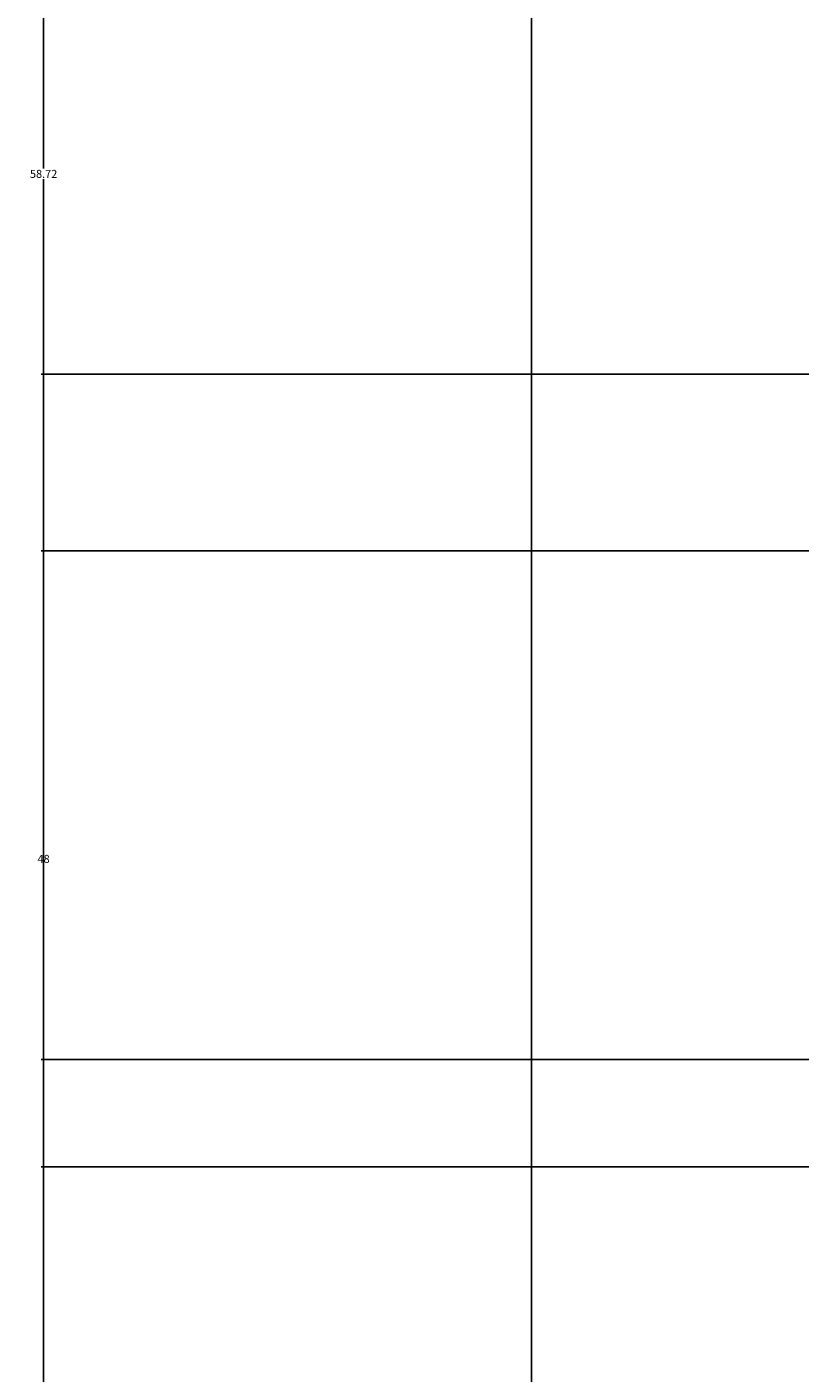
# Model space of a CAD drawing. Units: inches. Extents: x -13 to 809, y 112 to 656.
# Tile 26 of 55: x -13 to 47, y 446 to 551. Entities that reach past the tile are written whole.
import ezdxf

# ---------------------------------------------------------------- set-up
doc = ezdxf.new("R2010")
doc.units = ezdxf.units.IN
doc.header["$MEASUREMENT"] = 0
doc.layers.add('A-ANNO-DIMS', color=2, linetype='Continuous', lineweight=18)
doc.styles.get("Standard").update_dxf_attribs({"font": 'arial.ttf'})
doc.dimstyles.get("Standard").update_dxf_attribs({"dimtxt": 0.625, "dimasz": 0.18, "dimexe": 0.18, "dimexo": 0.0625, "dimgap": 0.09, "dimtad": 0, "dimtih": 1, "dimtoh": 1, "dimdec": 4, "dimzin": 0, "dimdsep": 46, "dimlunit": 4, "dimtxsty": 'Standard', "dimcen": 0.09, "dimadec": 0, "dimazin": 0, "dimtfac": 1, "dimtdec": 4, "dimtofl": 0, "dimtmove": 0, "dimatfit": 3, "dimfxl": 1, "dimtolj": 1, "dimtzin": 0, "dimarcsym": 0})

# ---------------------------------------------------------------- blocks, each defined once
blk = doc.blocks.new('*D22')
at = {"layer": 'A-ANNO-DIMS', "color": 0, "lineweight": -2, "transparency": 16777216}
for p, q in [((26.08, 210.58), (26.08, 655.96)), ((26.26, 655.78), (65.52, 655.78)), ((107.08, 655.78), (67.82, 655.78)), ((107.26, 510.58), (107.26, 655.96))]:
    blk.add_line(p, q, dxfattribs=at)
at = {"layer": 'A-ANNO-DIMS', "color": 0, "transparency": 16777216}
for points in [[(26.26, 655.81), (26.26, 655.75), (26.08, 655.78)], [(107.08, 655.81), (107.08, 655.75), (107.26, 655.78)]]:
    blk.add_solid(points, dxfattribs=at)
at = {"layer": 'Defpoints', "color": 0, "transparency": 16777216}
for p in [(107.26, 655.78), (107.26, 510.52), (26.08, 210.52)]:
    blk.add_point(p, dxfattribs=at)
at = {"layer": 'A-ANNO-DIMS', "color": 0, "transparency": 16777216, "insert": (66.67, 655.78), "char_height": 0.625, "attachment_point": 5}
blk.add_mtext('\\A1;81.18', dxfattribs=at)
blk = doc.blocks.new('*D34')
at = {"layer": 'A-ANNO-DIMS', "color": 0, "lineweight": -2, "transparency": 16777216}
for p, q in [((94.98, 462.52), (-12.1, 462.52)), ((-11.92, 462.34), (-11.92, 384.93)), ((-11.92, 306.7), (-11.92, 384.11)), ((94.98, 306.52), (-12.1, 306.52))]:
    blk.add_line(p, q, dxfattribs=at)
at = {"layer": 'A-ANNO-DIMS', "color": 0, "transparency": 16777216}
for points in [[(-11.95, 462.34), (-11.89, 462.34), (-11.92, 462.52)], [(-11.95, 306.7), (-11.89, 306.7), (-11.92, 306.52)]]:
    blk.add_solid(points, dxfattribs=at)
at = {"layer": 'Defpoints', "color": 0, "transparency": 16777216}
for p in [(-11.92, 462.52), (95.05, 462.52), (95.05, 306.52)]:
    blk.add_point(p, dxfattribs=at)
at = {"layer": 'A-ANNO-DIMS', "color": 0, "transparency": 16777216, "insert": (-11.92, 384.52), "char_height": 0.625, "attachment_point": 5}
blk.add_mtext('\\A1;156', dxfattribs=at)
blk = doc.blocks.new('*D35')
at = {"layer": 'A-ANNO-DIMS', "color": 0, "lineweight": -2, "transparency": 16777216}
for p, q in [((107.2, 510.52), (-12.1, 510.52)), ((-11.92, 510.34), (-11.92, 486.93)), ((-11.92, 462.7), (-11.92, 486.11)), ((107.2, 462.52), (-12.1, 462.52))]:
    blk.add_line(p, q, dxfattribs=at)
at = {"layer": 'A-ANNO-DIMS', "color": 0, "transparency": 16777216}
for points in [[(-11.95, 510.34), (-11.89, 510.34), (-11.92, 510.52)], [(-11.95, 462.7), (-11.89, 462.7), (-11.92, 462.52)]]:
    blk.add_solid(points, dxfattribs=at)
at = {"layer": 'Defpoints', "color": 0, "transparency": 16777216}
for p in [(-11.92, 510.52), (107.26, 510.52), (107.26, 462.52)]:
    blk.add_point(p, dxfattribs=at)
at = {"layer": 'A-ANNO-DIMS', "color": 0, "transparency": 16777216, "insert": (-11.92, 486.52), "char_height": 0.625, "attachment_point": 5}
blk.add_mtext('\\A1;48', dxfattribs=at)
blk = doc.blocks.new('*D36')
at = {"layer": 'A-ANNO-DIMS', "color": 0, "lineweight": -2, "transparency": 16777216}
for p, q in [((311.64, 569.24), (-12.1, 569.24)), ((-11.92, 569.06), (-11.92, 540.29)), ((-11.92, 510.7), (-11.92, 539.47)), ((107.2, 510.52), (-12.1, 510.52))]:
    blk.add_line(p, q, dxfattribs=at)
at = {"layer": 'A-ANNO-DIMS', "color": 0, "transparency": 16777216}
for points in [[(-11.95, 569.06), (-11.89, 569.06), (-11.92, 569.24)], [(-11.95, 510.7), (-11.89, 510.7), (-11.92, 510.52)]]:
    blk.add_solid(points, dxfattribs=at)
at = {"layer": 'Defpoints', "color": 0, "transparency": 16777216}
for p in [(-11.92, 569.24), (311.7, 569.24), (107.26, 510.52)]:
    blk.add_point(p, dxfattribs=at)
at = {"layer": 'A-ANNO-DIMS', "color": 0, "transparency": 16777216, "insert": (-11.92, 539.88), "char_height": 0.625, "attachment_point": 5}
blk.add_mtext('\\A1;58.72', dxfattribs=at)
blk = doc.blocks.new('*D39')
at = {"layer": 'A-ANNO-DIMS', "color": 0, "lineweight": -2, "transparency": 16777216}
for p, q in [((341.34, 524.28), (-12.1, 524.28)), ((-11.92, 524.1), (-11.92, 406.78)), ((-11.92, 288.63), (-11.92, 405.96)), ((341.34, 288.45), (-12.1, 288.45))]:
    blk.add_line(p, q, dxfattribs=at)
at = {"layer": 'A-ANNO-DIMS', "color": 0, "transparency": 16777216}
for points in [[(-11.95, 524.1), (-11.89, 524.1), (-11.92, 524.28)], [(-11.95, 288.63), (-11.89, 288.63), (-11.92, 288.45)]]:
    blk.add_solid(points, dxfattribs=at)
at = {"layer": 'Defpoints', "color": 0, "transparency": 16777216}
for p in [(-11.92, 524.28), (341.41, 524.28), (341.41, 288.45)]:
    blk.add_point(p, dxfattribs=at)
at = {"layer": 'A-ANNO-DIMS', "color": 0, "transparency": 16777216, "insert": (-11.92, 406.37), "char_height": 0.625, "attachment_point": 5}
blk.add_mtext('\\A1;235.83', dxfattribs=at)
blk = doc.blocks.new('*D43')
at = {"layer": 'A-ANNO-DIMS', "color": 0, "lineweight": -2, "transparency": 16777216}
for p, q in [((471.04, 470.88), (-12.1, 470.88)), ((-11.92, 470.7), (-11.92, 443.28)), ((-11.92, 415.04), (-11.92, 442.46)), ((471.04, 414.86), (-12.1, 414.86))]:
    blk.add_line(p, q, dxfattribs=at)
at = {"layer": 'A-ANNO-DIMS', "color": 0, "transparency": 16777216}
for points in [[(-11.95, 470.7), (-11.89, 470.7), (-11.92, 470.88)], [(-11.95, 415.04), (-11.89, 415.04), (-11.92, 414.86)]]:
    blk.add_solid(points, dxfattribs=at)
at = {"layer": 'Defpoints', "color": 0, "transparency": 16777216}
for p in [(-11.92, 470.88), (471.1, 470.88), (471.1, 414.86)]:
    blk.add_point(p, dxfattribs=at)
at = {"layer": 'A-ANNO-DIMS', "color": 0, "transparency": 16777216, "insert": (-11.92, 442.87), "char_height": 0.625, "attachment_point": 5}
blk.add_mtext('\\A1;56.02', dxfattribs=at)

msp = doc.modelspace()

# ---------------------------------------------------------------- dimensions: what is measured, and where the dimension line sits
at = {"layer": 'A-ANNO-DIMS'}
dim = msp.add_linear_dim(base=(107.2588, 655.7828), p1=(26.0809, 210.5199), p2=(107.2588, 510.5199), dimstyle='Standard', override={"dimdec": 2, "dimlfac": 1, "dimrnd": 0, "dimzin": 0, "dimdsep": 46, "dimlunit": 2}, dxfattribs=at)
dim.commit()
dim.dimension.update_dxf_attribs({"geometry": '*D22', "text_midpoint": (66.6698, 655.7828)})
for base, p1, p2, override, picture, middle in [((-11.9191, 569.2414), (107.2588, 510.5199), (311.6991, 569.2414), {"dimdec": 2, "dimlfac": 1, "dimrnd": 0, "dimzin": 0, "dimdsep": 46, "dimlunit": 2}, '*D36', (-11.9191, 539.8806)), ((-11.9191, 524.281), (341.4072, 288.4508), (341.4072, 524.281), {"dimdec": 2, "dimlfac": 1, "dimrnd": 0, "dimzin": 0, "dimdsep": 46, "dimlunit": 2}, '*D39', (-11.9191, 406.3659)), ((-11.9191, 510.5199), (107.2588, 462.5199), (107.2588, 510.5199), {"dimdec": 0, "dimlfac": 1, "dimrnd": 0, "dimzin": 0, "dimdsep": 46, "dimlunit": 2}, '*D35', (-11.9191, 486.5199)), ((-11.9191, 470.8765), (471.0998, 414.8594), (471.0998, 470.8765), {"dimdec": 2, "dimlfac": 1, "dimrnd": 0, "dimzin": 0, "dimdsep": 46, "dimlunit": 2}, '*D43', (-11.9191, 442.8679)), ((-11.9191, 462.5199), (95.0469, 306.5199), (95.0469, 462.5199), {"dimdec": 0, "dimlfac": 1, "dimrnd": 0, "dimzin": 0, "dimdsep": 46, "dimlunit": 2}, '*D34', (-11.9191, 384.5199))]:
    dim = msp.add_linear_dim(base=base, p1=p1, p2=p2, angle=90, dimstyle='Standard', override=override, dxfattribs=at)
    dim.commit()
    dim.dimension.update_dxf_attribs({"geometry": picture, "text_midpoint": middle})

doc.saveas('drawing.dxf')
